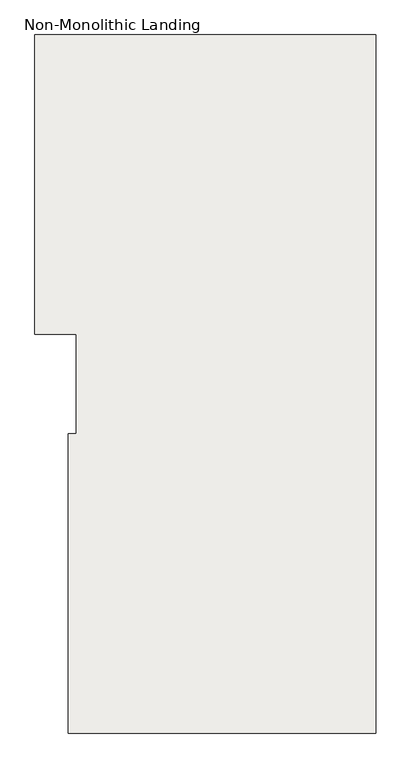
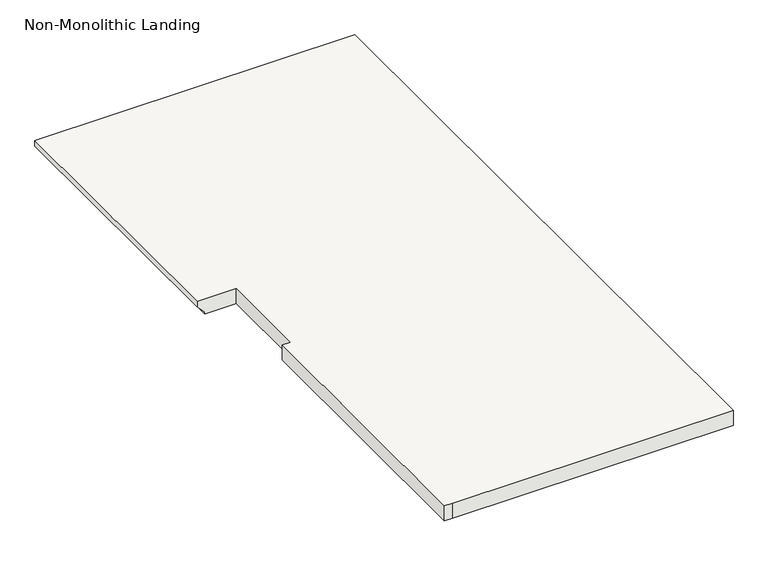
"""IFC4 building model written with IfcOpenShell, lengths in millimetres: slab geometry, Non-Monolithic Landing."""

from ifc_helpers import new_model, si_unit, origin, place, context, project, spatial, faceted_brep, source, transform, mapped, element, save


def non_monolithic_landing_b58457b6(model_context):
    return source(origin(), model_context, "Body", "Brep", [
        faceted_brep([(551.235938, 2339.7857363, 7888.8166667), (551.235938, 2339.7857363, 7907.8666667), (551.235938, 3254.1857363, 7907.8666667), (551.235938, 3254.1857363, 7888.8166667), (576.635938, 2339.7857363, 7863.4166667), (576.635938, 3254.1857363, 7863.4166667), (678.235938, 2339.7857363, 7907.8666667), (678.235938, 2034.9857363, 7907.8666667), (652.835938, 2034.9857363, 7907.8666667), (652.835938, 1120.5857363, 7907.8666667), (678.235938, 1120.5857363, 7907.8666667), (1592.635938, 1120.5857363, 7907.8666667), (1592.635938, 3254.1857363, 7907.8666667), (576.635938, 2339.7857363, 7857.0666667), (576.635938, 3254.1857363, 7857.0666667), (1592.635938, 3254.1857363, 7857.0666667), (1592.635938, 1120.5857363, 7857.0666667), (678.235938, 1120.5857363, 7857.0666667), (652.835938, 1120.5857363, 7857.0666667), (652.835938, 2034.9857363, 7857.0666667), (678.235938, 2034.9857363, 7857.0666667), (678.235938, 2339.7857363, 7857.0666667)], [[[0, 1, 2, 3]], [[4, 0, 3, 5]], [[6, 7, 8, 9, 10, 11, 12, 2, 1]], [[13, 14, 15, 16, 17, 18, 19, 20, 21]], [[14, 13, 4, 5]], [[6, 1, 0, 4, 13, 21]], [[7, 6, 21, 20]], [[8, 7, 20, 19]], [[9, 8, 19, 18]], [[10, 9, 18, 17]], [[11, 10, 17, 16]], [[12, 11, 16, 15]], [[2, 12, 15, 14, 5, 3]]]),
    ])


if __name__ == "__main__":
    model = new_model("IFC4")
    model_context = context("Model", 3, world=origin())
    ifc_project = project(units=[si_unit("LENGTHUNIT", "METRE", prefix="MILLI")], contexts=[model_context])
    site = spatial("IfcSite", under=ifc_project)
    building = spatial("IfcBuilding", under=site)
    placement = place(None, origin())
    non_monolithic_landing_shape = non_monolithic_landing_b58457b6(model_context)
    element("IfcSlab", 1, ObjectType="Non-Monolithic Landing", at=placement, inside=building, context=model_context, shape_type="MappedRepresentation", body=[
        mapped(non_monolithic_landing_shape, transform((0.0, 0.0, 0.0), x_axis=(1.0, 0.0, 0.0), y_axis=(0.0, 1.0, 0.0), z_axis=(0.0, 0.0, 1.0))),
    ])
    save(model, "model.ifc")

# Revit data of these elements
# Element 1 (IfcSlab, "Non-Monolithic Landing")
#   Materials on its faces: "BURGUNDY COLOUR"
# Materials
#   "BURGUNDY COLOUR": class "Generic", colour RGB 120 120 120, transparency 0, Cost = 0
